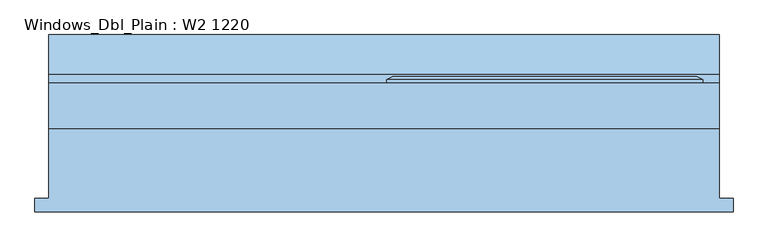
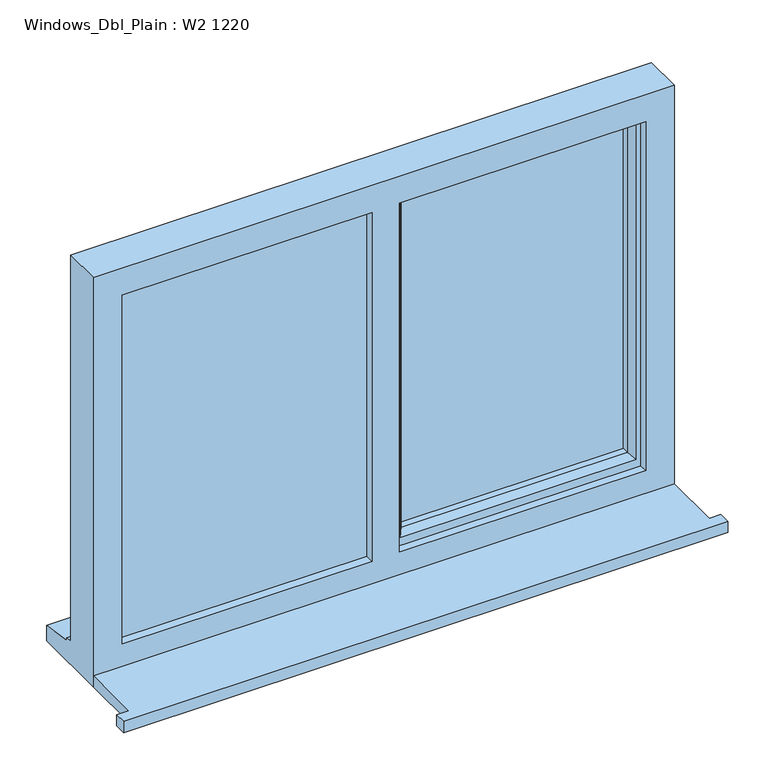
"""IFC4 building model written with IfcOpenShell, lengths in millimetres: window geometry, Windows_Dbl_Plain : W2 1220."""

from ifc_helpers import new_model, si_unit, frame, origin, place, context, project, spatial, polyline, outline, extrude, faceted_brep, source, transform, mapped, element, save


def windows_dbl_plain_w2_1220_793197e7(model_context):
    return source(origin(), model_context, "Body", "SolidModel", [
        extrude(outline(polyline([(-920.0, -146.5434322), (-920.0, -121.5434322), (-895.0, -121.5434322), (-895.0, 5.4565678), (325.0, 5.4565678), (325.0, -121.5434322), (350.0, -121.5434322), (350.0, -146.5434322), (-920.0, -146.5434322)])), frame((0.0, 0.0, 1200.0), z_axis=(0.0, 0.0, 1.0), x_axis=(1.0, 0.0, 0.0)), (0.0, 0.0, 1.0), 25.0),
        faceted_brep([(-280.0, 88.4565678, 2080.0), (-280.0, 94.2300705, 2080.0), (-280.0, 94.2300705, 1253.0), (-280.0, 88.4565678, 1253.0), (-270.0, 23.4565678, 2070.0), (-270.0, 88.4565678, 2070.0), (-270.0, 88.4565678, 1263.0), (-270.0, 23.4565678, 1263.0), (-230.0, 37.9494677, 2030.0), (-240.1480377, 23.4565678, 2040.1480377), (-240.1480377, 23.4565678, 1292.8519623), (-230.0, 37.9494677, 1303.0), (-230.0, 52.4565678, 2030.0), (-230.0, 52.4565678, 1303.0), (-240.0, 76.4565678, 2040.0), (-240.0, 52.4565678, 2040.0), (-240.0, 52.4565678, 1293.0), (-240.0, 76.4565678, 1293.0), (-230.0, 94.2300705, 2030.0), (-230.0, 76.4565678, 2030.0), (-230.0, 76.4565678, 1303.0), (-230.0, 94.2300705, 1303.0), (-247.4457548, 100.0035732, 2047.4457548), (-247.4457548, 100.0035732, 1285.5542452), (-269.2153903, 100.0035732, 2069.2153903), (-269.2153903, 100.0035732, 1263.7846097), (295.0, 94.2300705, 1253.0), (295.0, 88.4565678, 1253.0), (285.0, 88.4565678, 1263.0), (285.0, 23.4565678, 1263.0), (255.1480377, 23.4565678, 1292.8519623), (245.0, 37.9494677, 1303.0), (245.0, 52.4565678, 1303.0), (255.0, 52.4565678, 1293.0), (255.0, 76.4565678, 1293.0), (245.0, 76.4565678, 1303.0), (245.0, 94.2300705, 1303.0), (262.4457548, 100.0035732, 1285.5542452), (284.2153903, 100.0035732, 1263.7846097), (295.0, 94.2300705, 2080.0), (295.0, 88.4565678, 2080.0), (285.0, 88.4565678, 2070.0), (285.0, 23.4565678, 2070.0), (255.1480377, 23.4565678, 2040.1480377), (245.0, 37.9494677, 2030.0), (245.0, 52.4565678, 2030.0), (255.0, 52.4565678, 2040.0), (255.0, 76.4565678, 2040.0), (245.0, 76.4565678, 2030.0), (245.0, 94.2300705, 2030.0), (262.4457548, 100.0035732, 2047.4457548), (284.2153903, 100.0035732, 2069.2153903)], [[[0, 1, 2, 3]], [[4, 5, 6, 7]], [[8, 9, 10, 11]], [[12, 8, 11, 13]], [[14, 15, 16, 17]], [[18, 19, 20, 21]], [[22, 18, 21, 23]], [[1, 24, 25, 2]], [[3, 2, 26, 27]], [[7, 6, 28, 29]], [[11, 10, 30, 31]], [[13, 11, 31, 32]], [[17, 16, 33, 34]], [[21, 20, 35, 36]], [[23, 21, 36, 37]], [[2, 25, 38, 26]], [[27, 26, 39, 40]], [[29, 28, 41, 42]], [[31, 30, 43, 44]], [[32, 31, 44, 45]], [[34, 33, 46, 47]], [[36, 35, 48, 49]], [[37, 36, 49, 50]], [[26, 38, 51, 39]], [[40, 39, 1, 0]], [[3, 27, 40, 0], [5, 41, 28, 6]], [[42, 41, 5, 4]], [[7, 29, 42, 4], [9, 43, 30, 10]], [[44, 43, 9, 8]], [[45, 44, 8, 12]], [[15, 46, 33, 16], [13, 32, 45, 12]], [[47, 46, 15, 14]], [[17, 34, 47, 14], [19, 48, 35, 20]], [[49, 48, 19, 18]], [[50, 49, 18, 22]], [[24, 51, 38, 25], [23, 37, 50, 22]], [[39, 51, 24, 1]]]),
        extrude(outline(polyline([(2050.0, -310.0), (2070.0, -310.0), (2070.0, -855.0), (1263.0, -855.0), (1263.0, -310.0), (1283.0, -310.0), (1283.0, -835.0), (2050.0, -835.0), (2050.0, -310.0)])), frame((0.0, 47.4565678, 0.0), z_axis=(0.0, 1.0, 0.0), x_axis=(0.0, 0.0, 1.0)), (0.0, 0.0, 1.0), 41.0),
        faceted_brep([(325.0, 5.4565678, 2110.0), (-895.0, 5.4565678, 2110.0), (-895.0, 5.4565678, 1200.0), (325.0, 5.4565678, 1200.0), (265.0, 5.4565678, 2050.0), (265.0, 5.4565678, 1275.0), (-252.0, 5.4565678, 1275.0), (-252.0, 5.4565678, 2050.0), (-310.0, 5.4565678, 2050.0), (-310.0, 5.4565678, 1275.0), (-835.0, 5.4565678, 1275.0), (-835.0, 5.4565678, 2050.0), (-895.0, 88.4565678, 2110.0), (-895.0, 88.4565678, 1251.0), (-895.0, 103.4565678, 1249.68767), (-895.0, 103.4565678, 1244.7449676), (-895.0, 175.9565678, 1233.8088847), (-895.0, 175.9565678, 1200.0), (325.0, 88.4565678, 2110.0), (325.0, 88.4565678, 1251.0), (-855.0, 88.4565678, 2070.0), (-855.0, 88.4565678, 1263.0), (-310.0, 88.4565678, 1263.0), (-310.0, 88.4565678, 2070.0), (-270.0, 88.4565678, 2070.0), (-270.0, 88.4565678, 1263.0), (285.0, 88.4565678, 1263.0), (285.0, 88.4565678, 2070.0), (-855.0, 23.4565678, 2070.0), (-855.0, 23.4565678, 1263.0), (-300.0, 23.4565678, 2070.0), (-300.0, 23.4565678, 1263.0), (-310.0, 23.4565678, 2050.0), (-835.0, 23.4565678, 2050.0), (-835.0, 23.4565678, 1275.0), (-310.0, 23.4565678, 1275.0), (-270.0, 23.4565678, 2070.0), (285.0, 23.4565678, 2070.0), (285.0, 23.4565678, 1263.0), (-270.0, 23.4565678, 1263.0), (265.0, 23.4565678, 2050.0), (-252.0, 23.4565678, 2050.0), (-252.0, 23.4565678, 1275.0), (265.0, 23.4565678, 1275.0), (-310.0, 47.4565678, 2070.0), (-300.0, 47.4565678, 2070.0), (325.0, 175.9565678, 1200.0), (325.0, 175.9565678, 1233.8088847), (325.0, 103.4565678, 1244.7449676), (325.0, 103.4565678, 1249.68767), (-300.0, 47.4565678, 1263.0), (-310.0, 47.4565678, 1263.0)], [[[0, 1, 2, 3], [4, 5, 6, 7], [8, 9, 10, 11]], [[2, 1, 12, 13, 14, 15, 16, 17]], [[13, 12, 18, 19], [20, 21, 22, 23], [24, 25, 26, 27]], [[21, 20, 28, 29]], [[28, 30, 31, 29], [32, 33, 34, 35]], [[36, 37, 38, 39], [40, 41, 42, 43]], [[33, 11, 10, 34]], [[1, 0, 18, 12]], [[28, 20, 23, 44, 45, 30]], [[27, 37, 36, 24]], [[11, 33, 32, 8]], [[40, 4, 7, 41]], [[19, 18, 0, 3, 46, 47, 48, 49]], [[27, 26, 38, 37]], [[4, 40, 43, 5]], [[45, 50, 31, 30]], [[50, 45, 44, 51]], [[51, 44, 23, 22]], [[25, 24, 36, 39]], [[41, 7, 6, 42]], [[8, 32, 35, 9]], [[46, 3, 2, 17]], [[47, 46, 17, 16]], [[48, 47, 16, 15]], [[49, 48, 15, 14]], [[19, 49, 14, 13]], [[22, 21, 29, 31, 50, 51]], [[26, 25, 39, 38]], [[6, 5, 43, 42]], [[35, 34, 10, 9]]]),
        extrude(outline(polyline([(-855.0, 47.4565678), (-300.0, 47.4565678), (-300.0, 23.4565678), (-855.0, 23.4565678), (-855.0, 47.4565678)])), frame((0.0, 0.0, 1263.0), z_axis=(0.0, 0.0, 1.0), x_axis=(1.0, 0.0, 0.0)), (0.0, 0.0, 1.0), 807.0),
        extrude(outline(polyline([(255.0, 52.4565678), (-240.0, 52.4565678), (-240.0, 76.4565678), (255.0, 76.4565678), (255.0, 52.4565678)])), frame((0.0, 0.0, 1293.0), z_axis=(0.0, 0.0, 1.0), x_axis=(1.0, 0.0, 0.0)), (0.0, 0.0, 1.0), 747.0),
    ])


if __name__ == "__main__":
    model = new_model("IFC4")
    model_context = context("Model", 3, world=origin())
    ifc_project = project(units=[si_unit("LENGTHUNIT", "METRE", prefix="MILLI")], contexts=[model_context])
    site = spatial("IfcSite", under=ifc_project)
    building = spatial("IfcBuilding", under=site)
    placement = place(None, origin())
    windows_dbl_plain_w2_1220_shape = windows_dbl_plain_w2_1220_793197e7(model_context)
    element("IfcWindow", 1, ObjectType="Windows_Dbl_Plain : W2 1220", at=placement, inside=building, context=model_context, shape_type="MappedRepresentation", body=[
        mapped(windows_dbl_plain_w2_1220_shape, transform((0.0, 0.0, 0.0), x_axis=(1.0, 0.0, 0.0), y_axis=(0.0, 1.0, 0.0), z_axis=(0.0, 0.0, 1.0))),
    ])
    save(model, "model.ifc")

# Revit data of these elements
# Type "Windows_Dbl_Plain : W2 1220"
#   Type Mark = "63"
#   Operation = "DoublePanelVertical"
#   Construction Type Id = "GSP4R"
#   Manufacturer = "Revit"
#   Keynote = "L10"
#   Analytic Construction = "1/8 in Pilkington single glazing"
#   Wrap Layers (Ext) from Ext = 102.5 mm
#   Wrap Layers (Int) from Ext = 177.5 mm
#   Window Board Projection = 25 mm
#   Window Board Extension = 25 mm
#   Visual Light Transmittance = 0.9
#   Solar Heat Gain Coefficient = 0.78
#   Rough Width = 1220 mm
#   Rough Height = 910 mm
#   Height = 910 mm
#   Width = 1220 mm
#   Heat Transfer Coefficient (U) = 3.6886 W/(m²·K)
#   Glazing Thickness = 24 mm
#   FrameOffset - External = 50 mm
#   Frame Depth = 65 mm
#   Default Head Height = 2110 mm
#   Cill Depth = 87.5 mm
#   Cavity Closer Width = 50 mm
#   Cavity Closer Offset from Ext = 102.5 mm
#   Cavity Closer Depth = 85 mm
#   Vis - Cavity Closers = yes
#   Define Thermal Properties by = 1
#   Material Trim = Window Frame
#   Material Glass = Glass
#   Material Frame = Window Frame
#   Wall Closure = (empty or 0)
# Element 1 (IfcWindow, "Windows_Dbl_Plain : W2 1220")
#   Materials on its faces: "Window Frame", "Glass"
# Materials
#   "Window Frame": colour RGB 249 249 249, transparency 0, Keynote = "L10", Cost = 0
#   "Glass": class "Glass", colour RGB 0 128 192, transparency 0.9, Description = "Soda Lime Glass", Cost = 0
